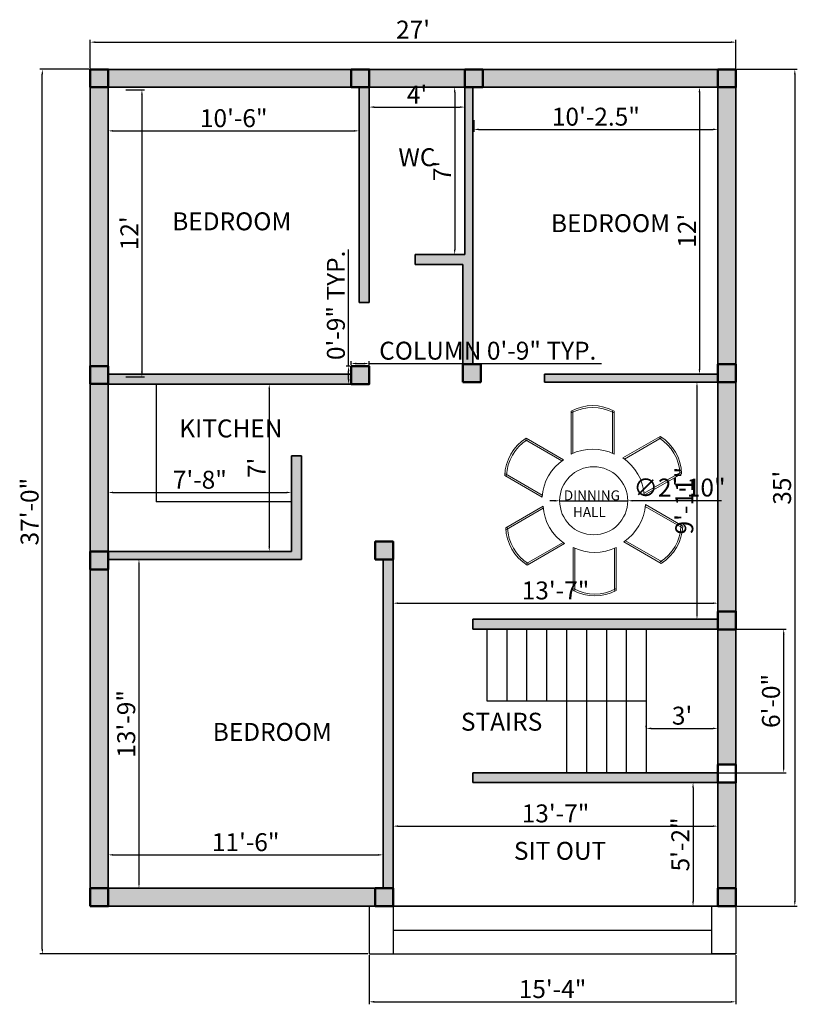
# Model space of a CAD drawing. Units: inches. Extents: x 1227 to 1617, y 420 to 915.
import ezdxf

# ---------------------------------------------------------------- set-up
doc = ezdxf.new("R2010")
doc.units = ezdxf.units.IN
for name, color, linetype, lineweight in [('A-ANNO-DIMS', 2, 'Continuous', 18), ('A-AREA-IDEN', 7, 'Continuous', 25), ('A-COLS', 7, 'Continuous', 50), ('A-FLOR-FIXT', 9, 'Continuous', 25), ('A-FLOR-STRS', 7, 'Continuous', 25), ('A-FURN', 8, 'Continuous', 18), ('A-WALL', 7, 'Continuous', 35)]:
    doc.layers.add(name, color=color, linetype=linetype, lineweight=lineweight)
doc.layers.add('A-COLS-PATT', color=18, linetype='Continuous', lineweight=13, true_color=0x000000)
doc.layers.add('A-WALL-PATT', color=114, linetype='Continuous', lineweight=13, true_color=0x139b48)
doc.styles.get("Standard").update_dxf_attribs({"font": 'arial.ttf'})
doc.dimstyles.new('ISO-25', dxfattribs={"dimtxt": 9, "dimasz": 2.5, "dimexe": 1.25, "dimexo": 0.625, "dimtad": 1, "dimlunit": 3, "dimtxsty": 'Standard', "dimcen": 2.5, "dimadec": 0, "dimazin": 0, "dimtfac": 1, "dimtmove": 0, "dimatfit": 3, "dimfxl": 1, "dimarcsym": 0})

# ---------------------------------------------------------------- blocks, each defined once
blk = doc.blocks.new('*U1')
for p, q in [((-10.82, -9.47), (-10.82, 12.17)), ((-9.92, -9.47), (-9.92, 11.75)), ((9.92, 11.75), (9.92, -9.47)), ((10.82, 12.17), (10.82, -9.47))]:
    blk.add_line(p, q)
for centre, radius, start, end in [((0, 33.94), 24.31, 243.5697, 296.4303), ((0, 10.82), 22.99, 241.9214, 298.0786), ((0, 10.82), 22.09, 241.9214, 298.0786)]:
    blk.add_arc(centre, radius, start, end)
blk = doc.blocks.new('*U2')
at = {"layer": 'A-FURN', "color": 0, "linetype": 'ByBlock', "lineweight": -2, "transparency": 16777216}
for p, rotation in [((1607.24, 674.24), 180), ((1638.29, 656.91), 120), ((1576.71, 656), 239.9999999999999), ((1577.23, 620.45), 300), ((1638.82, 621.36), 59.99999999999999)]:
    blk.add_blockref('*U1', p, dxfattribs=dict(at, rotation=rotation))
blk.add_blockref('*U1', (1608.29, 603.12), dxfattribs=at)
blk = doc.blocks.new('*D3')
at = {"layer": 'A-ANNO-DIMS', "color": 0, "lineweight": -2, "transparency": 16777216}
for p, q in [((1279.83, 879.38), (1289.21, 879.38)), ((1287.96, 876.88), (1287.96, 737.88)), ((1279.83, 735.38), (1289.21, 735.38))]:
    blk.add_line(p, q, dxfattribs=at)
at = {"layer": 'A-ANNO-DIMS', "color": 0, "transparency": 16777216}
for points in [[(1287.54, 876.88), (1288.38, 876.88), (1287.96, 879.38)], [(1287.54, 737.88), (1288.38, 737.88), (1287.96, 735.38)]]:
    blk.add_solid(points, dxfattribs=at)
at = {"layer": 'Defpoints', "color": 0, "transparency": 16777216}
for p in [(1279.2, 879.38), (1279.2, 735.38), (1287.96, 735.38)]:
    blk.add_point(p, dxfattribs=at)
at = {"layer": 'A-ANNO-DIMS', "color": 0, "transparency": 16777216, "insert": (1282.82, 807.38), "char_height": 9, "attachment_point": 5, "rotation": 90}
blk.add_mtext("12'", dxfattribs=at)
blk = doc.blocks.new('*D4')
at = {"layer": 'A-ANNO-DIMS', "color": 0, "lineweight": -2, "transparency": 16777216}
for p, q in [((1271.02, 868.89), (1271.02, 857.54)), ((1397.02, 868.89), (1397.02, 857.54)), ((1273.52, 858.79), (1394.52, 858.79))]:
    blk.add_line(p, q, dxfattribs=at)
at = {"layer": 'A-ANNO-DIMS', "color": 0, "transparency": 16777216}
for points in [[(1273.52, 859.21), (1273.52, 858.38), (1271.02, 858.79)], [(1394.52, 859.21), (1394.52, 858.38), (1397.02, 858.79)]]:
    blk.add_solid(points, dxfattribs=at)
at = {"layer": 'Defpoints', "color": 0, "transparency": 16777216}
for p in [(1271.02, 869.52), (1397.02, 869.52), (1397.02, 858.79)]:
    blk.add_point(p, dxfattribs=at)
at = {"layer": 'A-ANNO-DIMS', "color": 0, "transparency": 16777216, "insert": (1334.02, 864.01), "char_height": 9, "attachment_point": 5}
blk.add_mtext('10\'-6"', dxfattribs=at)
blk = doc.blocks.new('*D5')
at = {"layer": 'A-ANNO-DIMS', "color": 0, "lineweight": -2, "transparency": 16777216}
for p, q in [((1402.02, 880.05), (1402.02, 869.48)), ((1450.02, 880.05), (1450.02, 869.48)), ((1404.52, 870.73), (1447.52, 870.73))]:
    blk.add_line(p, q, dxfattribs=at)
at = {"layer": 'A-ANNO-DIMS', "color": 0, "transparency": 16777216}
for points in [[(1404.52, 871.15), (1404.52, 870.31), (1402.02, 870.73)], [(1447.52, 871.15), (1447.52, 870.31), (1450.02, 870.73)]]:
    blk.add_solid(points, dxfattribs=at)
at = {"layer": 'Defpoints', "color": 0, "transparency": 16777216}
for p in [(1402.02, 880.68), (1450.02, 880.68), (1450.02, 870.73)]:
    blk.add_point(p, dxfattribs=at)
at = {"layer": 'A-ANNO-DIMS', "color": 0, "transparency": 16777216, "insert": (1426.02, 875.86), "char_height": 9, "attachment_point": 5}
blk.add_mtext("4'", dxfattribs=at)
blk = doc.blocks.new('*D6')
at = {"layer": 'A-ANNO-DIMS', "color": 0, "lineweight": -2, "transparency": 16777216}
for p, q in [((1449.4, 880.68), (1443.67, 880.68)), ((1444.92, 878.18), (1444.92, 799.18)), ((1449.4, 796.68), (1443.67, 796.68))]:
    blk.add_line(p, q, dxfattribs=at)
at = {"layer": 'A-ANNO-DIMS', "color": 0, "transparency": 16777216}
for points in [[(1444.51, 878.18), (1445.34, 878.18), (1444.92, 880.68)], [(1444.51, 799.18), (1445.34, 799.18), (1444.92, 796.68)]]:
    blk.add_solid(points, dxfattribs=at)
at = {"layer": 'Defpoints', "color": 0, "transparency": 16777216}
for p in [(1450.02, 880.68), (1444.92, 796.68), (1450.02, 796.68)]:
    blk.add_point(p, dxfattribs=at)
at = {"layer": 'A-ANNO-DIMS', "color": 0, "transparency": 16777216, "insert": (1439.8, 838.68), "char_height": 9, "attachment_point": 5, "rotation": 90}
blk.add_mtext("7'", dxfattribs=at)
blk = doc.blocks.new('*D7')
at = {"layer": 'A-ANNO-DIMS', "color": 0, "lineweight": -2, "transparency": 16777216}
for p, q in [((1454.52, 864.22), (1454.52, 858.28)), ((1577.02, 864.22), (1577.02, 858.28)), ((1457.02, 859.53), (1574.52, 859.53))]:
    blk.add_line(p, q, dxfattribs=at)
at = {"layer": 'A-ANNO-DIMS', "color": 0, "transparency": 16777216}
for points in [[(1457.02, 859.95), (1457.02, 859.12), (1454.52, 859.53)], [(1574.52, 859.95), (1574.52, 859.12), (1577.02, 859.53)]]:
    blk.add_solid(points, dxfattribs=at)
at = {"layer": 'Defpoints', "color": 0, "transparency": 16777216}
for p in [(1454.52, 864.85), (1577.02, 864.85), (1577.02, 859.53)]:
    blk.add_point(p, dxfattribs=at)
at = {"layer": 'A-ANNO-DIMS', "color": 0, "transparency": 16777216, "insert": (1515.77, 864.75), "char_height": 9, "attachment_point": 5}
blk.add_mtext('10\'-2.5"', dxfattribs=at)
blk = doc.blocks.new('*D8')
at = {"layer": 'A-ANNO-DIMS', "color": 0, "lineweight": -2, "transparency": 16777216}
for p, q in [((1576.4, 880.68), (1566.51, 880.68)), ((1567.76, 878.18), (1567.76, 739.18)), ((1576.35, 736.68), (1566.51, 736.68))]:
    blk.add_line(p, q, dxfattribs=at)
at = {"layer": 'A-ANNO-DIMS', "color": 0, "transparency": 16777216}
for points in [[(1567.35, 878.18), (1568.18, 878.18), (1567.76, 880.68)], [(1567.35, 739.18), (1568.18, 739.18), (1567.76, 736.68)]]:
    blk.add_solid(points, dxfattribs=at)
at = {"layer": 'Defpoints', "color": 0, "transparency": 16777216}
for p in [(1577.02, 880.68), (1567.76, 736.68), (1576.97, 736.68)]:
    blk.add_point(p, dxfattribs=at)
at = {"layer": 'A-ANNO-DIMS', "color": 0, "transparency": 16777216, "insert": (1562.62, 808.68), "char_height": 9, "attachment_point": 5, "rotation": 90}
blk.add_mtext("12'", dxfattribs=at)
blk = doc.blocks.new('*D9')
at = {"layer": 'A-ANNO-DIMS', "color": 0, "lineweight": -2, "transparency": 16777216}
for p, q in [((1352.49, 731.68), (1353.11, 731.68)), ((1351.86, 729.18), (1351.86, 650.18)), ((1352.49, 647.68), (1353.11, 647.68))]:
    blk.add_line(p, q, dxfattribs=at)
at = {"layer": 'A-ANNO-DIMS', "color": 0, "transparency": 16777216}
for points in [[(1351.45, 729.18), (1352.28, 729.18), (1351.86, 731.68)], [(1351.45, 650.18), (1352.28, 650.18), (1351.86, 647.68)]]:
    blk.add_solid(points, dxfattribs=at)
at = {"layer": 'Defpoints', "color": 0, "transparency": 16777216}
for p in [(1351.86, 731.68), (1351.86, 647.68), (1351.86, 647.68)]:
    blk.add_point(p, dxfattribs=at)
at = {"layer": 'A-ANNO-DIMS', "color": 0, "transparency": 16777216, "insert": (1346.74, 689.68), "char_height": 9, "attachment_point": 5, "rotation": 90}
blk.add_mtext("7'", dxfattribs=at)
blk = doc.blocks.new('*D10')
at = {"layer": 'A-ANNO-DIMS', "color": 0, "lineweight": -2, "transparency": 16777216}
for p, q in [((1271.02, 674.75), (1271.02, 678.56)), ((1273.52, 677.31), (1360.52, 677.31)), ((1363.02, 674.75), (1363.02, 678.56))]:
    blk.add_line(p, q, dxfattribs=at)
at = {"layer": 'A-ANNO-DIMS', "color": 0, "transparency": 16777216}
for points in [[(1273.52, 677.73), (1273.52, 676.9), (1271.02, 677.31)], [(1360.52, 677.73), (1360.52, 676.9), (1363.02, 677.31)]]:
    blk.add_solid(points, dxfattribs=at)
at = {"layer": 'Defpoints', "color": 0, "transparency": 16777216}
for p in [(1363.02, 677.31), (1271.02, 674.12), (1363.02, 674.12)]:
    blk.add_point(p, dxfattribs=at)
at = {"layer": 'A-ANNO-DIMS', "color": 0, "transparency": 16777216, "insert": (1317.02, 682.53), "char_height": 9, "attachment_point": 5}
blk.add_mtext('7\'-8"', dxfattribs=at)
blk = doc.blocks.new('*D11')
at = {"layer": 'A-ANNO-DIMS', "color": 0, "lineweight": -2, "transparency": 16777216}
for p, q in [((1287.1, 643.68), (1287.72, 643.68)), ((1286.47, 641.18), (1286.47, 481.18)), ((1287.1, 478.68), (1287.72, 478.68))]:
    blk.add_line(p, q, dxfattribs=at)
at = {"layer": 'A-ANNO-DIMS', "color": 0, "transparency": 16777216}
for points in [[(1286.06, 641.18), (1286.89, 641.18), (1286.47, 643.68)], [(1286.06, 481.18), (1286.89, 481.18), (1286.47, 478.68)]]:
    blk.add_solid(points, dxfattribs=at)
at = {"layer": 'Defpoints', "color": 0, "transparency": 16777216}
for p in [(1286.47, 643.68), (1286.47, 478.68), (1286.47, 478.68)]:
    blk.add_point(p, dxfattribs=at)
at = {"layer": 'A-ANNO-DIMS', "color": 0, "transparency": 16777216, "insert": (1281.25, 561.18), "char_height": 9, "attachment_point": 5, "rotation": 90}
blk.add_mtext('13\'-9"', dxfattribs=at)
blk = doc.blocks.new('*D12')
at = {"layer": 'A-ANNO-DIMS', "color": 0, "lineweight": -2, "transparency": 16777216}
for p, q in [((1271.02, 491.5), (1271.02, 496.67)), ((1273.52, 495.42), (1406.52, 495.42)), ((1409.02, 491.5), (1409.02, 496.67))]:
    blk.add_line(p, q, dxfattribs=at)
at = {"layer": 'A-ANNO-DIMS', "color": 0, "transparency": 16777216}
for points in [[(1273.52, 495.84), (1273.52, 495), (1271.02, 495.42)], [(1406.52, 495.84), (1406.52, 495), (1409.02, 495.42)]]:
    blk.add_solid(points, dxfattribs=at)
at = {"layer": 'Defpoints', "color": 0, "transparency": 16777216}
for p in [(1409.02, 495.42), (1271.02, 490.87), (1409.02, 490.87)]:
    blk.add_point(p, dxfattribs=at)
at = {"layer": 'A-ANNO-DIMS', "color": 0, "transparency": 16777216, "insert": (1340.02, 500.64), "char_height": 9, "attachment_point": 5}
blk.add_mtext('11\'-6"', dxfattribs=at)
blk = doc.blocks.new('*D13')
at = {"layer": 'A-ANNO-DIMS', "color": 0, "lineweight": -2, "transparency": 16777216}
for p, q in [((1541.02, 559.52), (1541.02, 560.14)), ((1543.52, 558.89), (1574.52, 558.89)), ((1577.02, 559.52), (1577.02, 560.14))]:
    blk.add_line(p, q, dxfattribs=at)
at = {"layer": 'A-ANNO-DIMS', "color": 0, "transparency": 16777216}
for points in [[(1543.52, 559.31), (1543.52, 558.47), (1541.02, 558.89)], [(1574.52, 559.31), (1574.52, 558.47), (1577.02, 558.89)]]:
    blk.add_solid(points, dxfattribs=at)
at = {"layer": 'Defpoints', "color": 0, "transparency": 16777216}
for p in [(1541.02, 558.89), (1577.02, 558.89), (1577.02, 558.89)]:
    blk.add_point(p, dxfattribs=at)
at = {"layer": 'A-ANNO-DIMS', "color": 0, "transparency": 16777216, "insert": (1559.02, 564.11), "char_height": 9, "attachment_point": 5}
blk.add_mtext("3'", dxfattribs=at)
blk = doc.blocks.new('*D14')
at = {"layer": 'A-ANNO-DIMS', "color": 0, "lineweight": -2, "transparency": 16777216}
for p, q in [((1564.54, 529.18), (1564.54, 472.18)), ((1565.16, 531.68), (1565.79, 531.68)), ((1565.16, 469.68), (1565.79, 469.68))]:
    blk.add_line(p, q, dxfattribs=at)
at = {"layer": 'A-ANNO-DIMS', "color": 0, "transparency": 16777216}
for points in [[(1564.12, 529.18), (1564.96, 529.18), (1564.54, 531.68)], [(1564.12, 472.18), (1564.96, 472.18), (1564.54, 469.68)]]:
    blk.add_solid(points, dxfattribs=at)
at = {"layer": 'Defpoints', "color": 0, "transparency": 16777216}
for p in [(1564.54, 531.68), (1564.54, 469.68), (1564.54, 469.68)]:
    blk.add_point(p, dxfattribs=at)
at = {"layer": 'A-ANNO-DIMS', "color": 0, "transparency": 16777216, "insert": (1559.32, 500.68), "char_height": 9, "attachment_point": 5, "rotation": 90}
blk.add_mtext('5\'-2"', dxfattribs=at)
blk = doc.blocks.new('*D15')
at = {"layer": 'A-ANNO-DIMS', "color": 0, "lineweight": -2, "transparency": 16777216}
for p, q in [((1414.02, 510.47), (1414.02, 511.09)), ((1416.52, 509.84), (1574.52, 509.84)), ((1577.02, 510.47), (1577.02, 511.09))]:
    blk.add_line(p, q, dxfattribs=at)
at = {"layer": 'A-ANNO-DIMS', "color": 0, "transparency": 16777216}
for points in [[(1416.52, 510.26), (1416.52, 509.43), (1414.02, 509.84)], [(1574.52, 510.26), (1574.52, 509.43), (1577.02, 509.84)]]:
    blk.add_solid(points, dxfattribs=at)
at = {"layer": 'Defpoints', "color": 0, "transparency": 16777216}
for p in [(1414.02, 509.84), (1577.02, 509.84), (1577.02, 509.84)]:
    blk.add_point(p, dxfattribs=at)
at = {"layer": 'A-ANNO-DIMS', "color": 0, "transparency": 16777216, "insert": (1495.52, 515.07), "char_height": 9, "attachment_point": 5}
blk.add_mtext('13\'-7"', dxfattribs=at)
blk = doc.blocks.new('*D16')
at = {"layer": 'A-ANNO-DIMS', "color": 0, "lineweight": -2, "transparency": 16777216}
for p, q in [((1414.02, 633.75), (1414.02, 620.5)), ((1577.02, 633.75), (1577.02, 620.5)), ((1416.52, 621.75), (1574.52, 621.75))]:
    blk.add_line(p, q, dxfattribs=at)
at = {"layer": 'A-ANNO-DIMS', "color": 0, "transparency": 16777216}
for points in [[(1416.52, 622.16), (1416.52, 621.33), (1414.02, 621.75)], [(1574.52, 622.16), (1574.52, 621.33), (1577.02, 621.75)]]:
    blk.add_solid(points, dxfattribs=at)
at = {"layer": 'Defpoints', "color": 0, "transparency": 16777216}
for p in [(1414.02, 634.38), (1577.02, 634.38), (1577.02, 621.75)]:
    blk.add_point(p, dxfattribs=at)
at = {"layer": 'A-ANNO-DIMS', "color": 0, "transparency": 16777216, "insert": (1495.52, 626.97), "char_height": 9, "attachment_point": 5}
blk.add_mtext('13\'-7"', dxfattribs=at)
blk = doc.blocks.new('*D17')
at = {"layer": 'A-ANNO-DIMS', "color": 0, "lineweight": -2, "transparency": 16777216}
for p, q in [((1567.14, 732.68), (1567.76, 732.68)), ((1566.51, 730.18), (1566.51, 616.18)), ((1567.14, 613.68), (1567.76, 613.68))]:
    blk.add_line(p, q, dxfattribs=at)
at = {"layer": 'A-ANNO-DIMS', "color": 0, "transparency": 16777216}
for points in [[(1566.1, 730.18), (1566.93, 730.18), (1566.51, 732.68)], [(1566.1, 616.18), (1566.93, 616.18), (1566.51, 613.68)]]:
    blk.add_solid(points, dxfattribs=at)
at = {"layer": 'Defpoints', "color": 0, "transparency": 16777216}
for p in [(1566.51, 732.68), (1566.51, 613.68), (1566.51, 613.68)]:
    blk.add_point(p, dxfattribs=at)
at = {"layer": 'A-ANNO-DIMS', "color": 0, "transparency": 16777216, "insert": (1561.29, 673.18), "char_height": 9, "attachment_point": 5, "rotation": 90}
blk.add_mtext('9\'-11"', dxfattribs=at)
blk = doc.blocks.new('*D18')
at = {"layer": 'A-ANNO-DIMS', "color": 0, "lineweight": -2, "transparency": 16777216}
for p, q in [((1262.02, 890.3), (1262.02, 904.56)), ((1586.02, 890.3), (1586.02, 904.56)), ((1264.52, 903.31), (1583.52, 903.31))]:
    blk.add_line(p, q, dxfattribs=at)
at = {"layer": 'A-ANNO-DIMS', "color": 0, "transparency": 16777216}
for points in [[(1264.52, 903.73), (1264.52, 902.9), (1262.02, 903.31)], [(1583.52, 903.73), (1583.52, 902.9), (1586.02, 903.31)]]:
    blk.add_solid(points, dxfattribs=at)
at = {"layer": 'Defpoints', "color": 0, "transparency": 16777216}
for p in [(1586.02, 903.31), (1262.02, 889.68), (1586.02, 889.68)]:
    blk.add_point(p, dxfattribs=at)
at = {"layer": 'A-ANNO-DIMS', "color": 0, "transparency": 16777216, "insert": (1424.02, 908.46), "char_height": 9, "attachment_point": 5}
blk.add_mtext("27'", dxfattribs=at)
blk = doc.blocks.new('*D19')
at = {"layer": 'A-ANNO-DIMS', "color": 0, "lineweight": -2, "transparency": 16777216}
for p, q in [((1586.65, 889.68), (1616.86, 889.68)), ((1615.61, 887.18), (1615.61, 472.18)), ((1586.65, 469.68), (1616.86, 469.68))]:
    blk.add_line(p, q, dxfattribs=at)
at = {"layer": 'A-ANNO-DIMS', "color": 0, "transparency": 16777216}
for points in [[(1615.19, 887.18), (1616.02, 887.18), (1615.61, 889.68)], [(1615.19, 472.18), (1616.02, 472.18), (1615.61, 469.68)]]:
    blk.add_solid(points, dxfattribs=at)
at = {"layer": 'Defpoints', "color": 0, "transparency": 16777216}
for p in [(1586.02, 889.68), (1586.02, 469.68), (1615.61, 469.68)]:
    blk.add_point(p, dxfattribs=at)
at = {"layer": 'A-ANNO-DIMS', "color": 0, "transparency": 16777216, "insert": (1610.38, 679.68), "char_height": 9, "attachment_point": 5, "rotation": 90}
blk.add_mtext("35'", dxfattribs=at)
blk = doc.blocks.new('COLUMN-9X9-IN')
blk.add_lwpolyline([(0, 0), (9, 0), (9, 9), (0, 9)], close=True)
blk = doc.blocks.new('*D21')
at = {"layer": 'A-ANNO-DIMS', "color": 0, "lineweight": -2, "transparency": 16777216}
for p, q in [((1393.02, 741.3), (1393.02, 743.28)), ((1395.52, 742.03), (1399.52, 742.03)), ((1402.02, 741.3), (1402.02, 743.28)), ((1402.02, 742.03), (1518.51, 742.03))]:
    blk.add_line(p, q, dxfattribs=at)
at = {"layer": 'A-ANNO-DIMS', "color": 0, "transparency": 16777216}
for points in [[(1395.52, 742.44), (1395.52, 741.61), (1393.02, 742.03)], [(1399.52, 742.44), (1399.52, 741.61), (1402.02, 742.03)]]:
    blk.add_solid(points, dxfattribs=at)
at = {"layer": 'Defpoints', "color": 0, "transparency": 16777216}
for p in [(1402.02, 742.03), (1393.02, 740.68), (1402.02, 740.68)]:
    blk.add_point(p, dxfattribs=at)
at = {"layer": 'A-ANNO-DIMS', "color": 0, "transparency": 16777216, "insert": (1461.51, 747.31), "char_height": 9, "attachment_point": 5}
blk.add_mtext('COLUMN 0\'-9" TYP.', dxfattribs=at)
blk = doc.blocks.new('*D22')
at = {"layer": 'A-ANNO-DIMS', "color": 0, "lineweight": -2, "transparency": 16777216}
for p, q in [((1391.67, 740.68), (1391.67, 799.29)), ((1392.4, 740.68), (1390.42, 740.68)), ((1391.67, 734.18), (1391.67, 738.18)), ((1392.4, 731.68), (1390.42, 731.68))]:
    blk.add_line(p, q, dxfattribs=at)
at = {"layer": 'A-ANNO-DIMS', "color": 0, "transparency": 16777216}
for points in [[(1391.26, 738.18), (1392.09, 738.18), (1391.67, 740.68)], [(1391.26, 734.18), (1392.09, 734.18), (1391.67, 731.68)]]:
    blk.add_solid(points, dxfattribs=at)
at = {"layer": 'Defpoints', "color": 0, "transparency": 16777216}
for p in [(1391.67, 740.68), (1393.02, 740.68), (1393.02, 731.68)]:
    blk.add_point(p, dxfattribs=at)
at = {"layer": 'A-ANNO-DIMS', "color": 0, "transparency": 16777216, "insert": (1386.45, 771.23), "char_height": 9, "attachment_point": 5, "rotation": 90}
blk.add_mtext('0\'-9" TYP.', dxfattribs=at)
blk = doc.blocks.new('*D23')
at = {"layer": 'A-ANNO-DIMS', "color": 0, "lineweight": -2, "transparency": 16777216}
for p, q in [((1402.02, 445.05), (1402.02, 420.43)), ((1586.02, 445.05), (1586.02, 420.43)), ((1404.52, 421.68), (1583.52, 421.68))]:
    blk.add_line(p, q, dxfattribs=at)
at = {"layer": 'A-ANNO-DIMS', "color": 0, "transparency": 16777216}
for points in [[(1404.52, 422.09), (1404.52, 421.26), (1402.02, 421.68)], [(1583.52, 422.09), (1583.52, 421.26), (1586.02, 421.68)]]:
    blk.add_solid(points, dxfattribs=at)
at = {"layer": 'Defpoints', "color": 0, "transparency": 16777216}
for p in [(1402.02, 445.68), (1586.02, 445.68), (1586.02, 421.68)]:
    blk.add_point(p, dxfattribs=at)
at = {"layer": 'A-ANNO-DIMS', "color": 0, "transparency": 16777216, "insert": (1494.02, 426.9), "char_height": 9, "attachment_point": 5}
blk.add_mtext('15\'-4"', dxfattribs=at)
blk = doc.blocks.new('*D24')
at = {"layer": 'A-ANNO-DIMS', "color": 0, "lineweight": -2, "transparency": 16777216}
for p, q in [((1577.65, 608.68), (1611.27, 608.68)), ((1610.02, 539.18), (1610.02, 606.18)), ((1577.65, 536.68), (1611.27, 536.68))]:
    blk.add_line(p, q, dxfattribs=at)
at = {"layer": 'A-ANNO-DIMS', "color": 0, "transparency": 16777216}
for points in [[(1609.61, 606.18), (1610.44, 606.18), (1610.02, 608.68)], [(1609.61, 539.18), (1610.44, 539.18), (1610.02, 536.68)]]:
    blk.add_solid(points, dxfattribs=at)
at = {"layer": 'Defpoints', "color": 0, "transparency": 16777216}
for p in [(1577.02, 608.68), (1610.02, 608.68), (1577.02, 536.68)]:
    blk.add_point(p, dxfattribs=at)
at = {"layer": 'A-ANNO-DIMS', "color": 0, "transparency": 16777216, "insert": (1604.8, 572.68), "char_height": 9, "attachment_point": 5, "rotation": 90}
blk.add_mtext('6\'-0"', dxfattribs=at)
blk = doc.blocks.new('*D25')
at = {"layer": 'A-ANNO-DIMS', "color": 0, "lineweight": -2, "transparency": 16777216}
for p, q in [((1261.4, 889.68), (1236.72, 889.68)), ((1237.97, 448.18), (1237.97, 887.18)), ((1401.4, 445.68), (1236.72, 445.68))]:
    blk.add_line(p, q, dxfattribs=at)
at = {"layer": 'A-ANNO-DIMS', "color": 0, "transparency": 16777216}
for points in [[(1237.56, 887.18), (1238.39, 887.18), (1237.97, 889.68)], [(1237.56, 448.18), (1238.39, 448.18), (1237.97, 445.68)]]:
    blk.add_solid(points, dxfattribs=at)
at = {"layer": 'Defpoints', "color": 0, "transparency": 16777216}
for p in [(1237.97, 889.68), (1262.02, 889.68), (1402.02, 445.68)]:
    blk.add_point(p, dxfattribs=at)
at = {"layer": 'A-ANNO-DIMS', "color": 0, "transparency": 16777216, "insert": (1232.75, 667.68), "char_height": 9, "attachment_point": 5, "rotation": 90}
blk.add_mtext('37\'-0"', dxfattribs=at)
blk = doc.blocks.new('*D26')
at = {"layer": 'A-ANNO-DIMS', "color": 0, "lineweight": -2, "transparency": 16777216}
for p, q in [((1495.09, 673.15), (1492.59, 673.15)), ((1497.59, 673.15), (1531.78, 673.15)), ((1578.74, 673.15), (1534.28, 673.15))]:
    blk.add_line(p, q, dxfattribs=at)
at = {"layer": 'A-ANNO-DIMS', "color": 0, "transparency": 16777216}
for points in [[(1495.09, 673.57), (1495.09, 672.73), (1497.59, 673.15)], [(1534.28, 673.57), (1534.28, 672.73), (1531.78, 673.15)]]:
    blk.add_solid(points, dxfattribs=at)
at = {"layer": 'Defpoints', "color": 0, "transparency": 16777216}
for p in [(1497.59, 673.15), (1531.78, 673.15)]:
    blk.add_point(p, dxfattribs=at)
at = {"layer": 'A-ANNO-DIMS', "color": 0, "transparency": 16777216, "insert": (1557.76, 678.62), "char_height": 9, "attachment_point": 5, "rotation": 0.001}
blk.add_mtext('∅2\'-10"', dxfattribs=at)

msp = doc.modelspace()

# ---------------------------------------------------------------- hatches: boundary and pattern name
at = {"layer": 'A-COLS-PATT'}
h = msp.add_hatch(color=256, dxfattribs=at)
h.dxf.hatch_style = 1
h.paths.add_polyline_path([(1271.023, 889.677), (1262.023, 889.677), (1262.023, 880.677), (1271.023, 880.677)])
h = msp.add_hatch(color=256, dxfattribs=at)
h.dxf.hatch_style = 1
h.paths.add_polyline_path([(1271.023, 478.677), (1262.023, 478.677), (1262.023, 469.677), (1271.023, 469.677)])
h.paths.add_polyline_path([(1414.023, 478.677), (1405.023, 478.677), (1405.023, 469.677), (1414.023, 469.677)])
h.paths.add_polyline_path([(1271.023, 647.677), (1262.023, 647.677), (1262.023, 638.677), (1271.023, 638.677)])
h.paths.add_polyline_path([(1402.023, 889.677), (1393.023, 889.677), (1393.023, 880.677), (1402.023, 880.677)])
h.paths.add_polyline_path([(1459.023, 889.677), (1450.023, 889.677), (1450.023, 880.677), (1459.023, 880.677)])
h.paths.add_polyline_path([(1586.023, 889.677), (1577.023, 889.677), (1577.023, 880.677), (1586.023, 880.677)])
h.paths.add_polyline_path([(1585.974, 741.727), (1577.023, 741.727), (1577.023, 736.677), (1576.974, 732.727), (1585.974, 732.727)])
h.paths.add_polyline_path([(1586.023, 617.607), (1577.023, 617.607), (1577.023, 608.607), (1586.023, 608.607)])
h.paths.add_polyline_path([(1414.023, 652.677), (1405.023, 652.677), (1405.023, 643.677), (1414.023, 643.677)])
h.paths.add_polyline_path([(1402.023, 740.677), (1393.023, 740.677), (1393.023, 731.677), (1402.023, 731.677)])
h.paths.add_polyline_path([(1458.015, 741.677), (1449.023, 741.677), (1449.023, 732.677), (1458.015, 732.677)])
h.paths.add_polyline_path([(1586.023, 478.677), (1577.023, 478.677), (1577.023, 469.677), (1586.023, 469.677)])
h.paths.add_polyline_path([(1270.972, 740.755), (1262.023, 740.755), (1262.023, 731.755), (1270.972, 731.755)])
at = {"layer": 'A-WALL-PATT'}
h = msp.add_hatch(color=256, dxfattribs=at)
h.dxf.hatch_style = 1
h.paths.add_polyline_path([(1262.023, 740.755), (1271.023, 740.755), (1271.023, 880.677), (1262.023, 880.677)])
h.paths.add_polyline_path([(1450.023, 880.677), (1450.023, 889.677), (1402.023, 889.677), (1402.023, 880.677)])
h.paths.add_polyline_path([(1577.023, 880.677), (1577.023, 889.677), (1459.023, 889.677), (1459.023, 880.677)])
h.paths.add_polyline_path([(1292.251, 796.549), (1292.251, 817.434), (1273.705, 817.434), (1273.705, 796.549)], flags=9)
h.paths.add_polyline_path([(1491.876, 855.398), (1538.89, 855.398), (1538.89, 873.944), (1491.876, 873.944)], flags=9)
h = msp.add_hatch(color=256, dxfattribs=at)
h.dxf.hatch_style = 1
h.paths.add_polyline_path([(1393.023, 889.677), (1271.023, 889.677), (1271.023, 880.677), (1393.023, 880.677)])
h.paths.add_polyline_path([(1393.023, 736.677), (1270.972, 736.677), (1270.972, 731.677), (1393.023, 731.677)])
h.paths.add_polyline_path([(1271.023, 731.677), (1270.972, 731.677), (1262.023, 731.754), (1262.023, 647.677), (1271.023, 647.677)])
h.paths.add_polyline_path([(1402.023, 880.677), (1397.023, 880.677), (1397.023, 772.677), (1402.023, 772.677)])
h.paths.add_polyline_path([(1454.023, 880.677), (1450.023, 880.677), (1450.023, 796.677), (1425.023, 796.677), (1425.023, 791.677), (1449.023, 791.677), (1449.023, 741.677), (1454.023, 741.677)])
h.paths.add_polyline_path([(1576.974, 736.677), (1490.023, 736.677), (1490.023, 732.677), (1576.974, 732.677)])
h.paths.add_polyline_path([(1586.023, 880.677), (1577.023, 880.677), (1577.023, 741.727), (1586.023, 741.727)])
h.paths.add_polyline_path([(1586.023, 608.607), (1577.023, 608.607), (1577.023, 540.743), (1586.023, 540.743)])
h.paths.add_polyline_path([(1586.023, 732.727), (1577.023, 732.727), (1577.023, 617.607), (1586.023, 617.607)])
h.paths.add_polyline_path([(1577.023, 613.677), (1454.023, 613.677), (1454.023, 608.677), (1577.023, 608.677)])
h.paths.add_polyline_path([(1577.023, 536.677), (1454.023, 536.677), (1454.023, 531.677), (1577.023, 531.677), (1577.023, 531.743)])
h.paths.add_polyline_path([(1586.023, 531.743), (1577.023, 531.743), (1577.023, 531.677), (1577.023, 478.677), (1586.023, 478.677)])
h.paths.add_polyline_path([(1405.023, 478.677), (1271.023, 478.677), (1271.023, 469.677), (1405.023, 469.677)])
h.paths.add_polyline_path([(1414.023, 643.677), (1409.023, 643.677), (1409.023, 478.677), (1414.023, 478.677)])
h.paths.add_polyline_path([(1271.023, 638.677), (1262.023, 638.677), (1262.023, 478.677), (1271.023, 478.677)])
h.paths.add_polyline_path([(1368.023, 695.677), (1363.023, 695.677), (1363.023, 647.677), (1271.023, 647.677), (1271.023, 643.677), (1367.023, 643.677), (1368.023, 643.677), (1368.023, 644.677)])

# ---------------------------------------------------------------- linework, layer by layer
at = {"layer": 'A-FLOR-FIXT'}
for p in [(1295.023, 731.677), (1363.023, 672.677)]:
    msp.add_line(p, (1295.023, 672.677), dxfattribs=at)
at = {"layer": 'A-FLOR-STRS'}
for p, q in [((1461.023, 608.677), (1461.023, 572.677)), ((1471.023, 608.677), (1471.023, 572.677)), ((1481.023, 608.677), (1481.023, 572.677)), ((1491.023, 608.677), (1491.023, 572.677)), ((1501.023, 608.677), (1501.023, 536.677)), ((1511.023, 608.677), (1511.023, 536.677)), ((1521.023, 608.677), (1521.023, 536.677)), ((1531.023, 608.677), (1531.023, 536.677)), ((1541.023, 608.677), (1541.023, 536.677)), ((1461.023, 572.677), (1541.023, 572.677)), ((1402.023, 469.677), (1402.023, 445.677)), ((1414.023, 469.677), (1414.023, 445.677)), ((1574.023, 445.677), (1574.023, 469.677)), ((1586.023, 469.677), (1586.023, 445.677)), ((1414.023, 457.677), (1574.023, 457.677)), ((1402.023, 445.677), (1426.023, 445.677)), ((1414.023, 445.677), (1586.023, 445.677)), ((1586.023, 445.677), (1574.023, 445.677))]:
    msp.add_line(p, q, dxfattribs=at)
at = {"layer": 'A-FURN'}
msp.add_circle((1514.683, 673.15), 17.097, dxfattribs=at)
at = {"layer": 'A-WALL'}
for p, q in [((1586.023, 889.677), (1262.023, 889.677)), ((1262.023, 889.677), (1262.023, 469.677)), ((1586.023, 469.677), (1586.023, 889.677)), ((1271.023, 880.677), (1271.023, 736.677)), ((1397.023, 880.677), (1271.023, 880.677)), ((1397.023, 880.677), (1397.023, 772.677)), ((1402.023, 880.677), (1402.023, 772.677)), ((1450.023, 880.677), (1402.023, 880.677)), ((1450.023, 880.677), (1450.023, 796.677)), ((1577.023, 880.677), (1454.023, 880.677)), ((1454.023, 880.677), (1454.023, 741.677)), ((1577.023, 736.677), (1577.023, 880.677)), ((1425.023, 796.677), (1449.023, 796.677)), ((1450.023, 796.677), (1425.023, 796.677)), ((1425.023, 796.677), (1425.023, 791.677)), ((1425.023, 791.677), (1449.023, 791.677)), ((1449.023, 791.677), (1449.023, 732.677)), ((1397.023, 772.677), (1402.023, 772.677)), ((1393.023, 736.677), (1271.023, 736.677)), ((1402.023, 731.677), (1402.023, 736.677)), ((1402.023, 736.677), (1402.023, 736.677)), ((1577.023, 736.677), (1490.023, 736.677)), ((1490.023, 736.677), (1490.023, 732.677)), ((1401.023, 731.677), (1271.023, 731.677)), ((1271.023, 731.677), (1271.023, 647.677)), ((1401.023, 731.677), (1402.023, 731.677)), ((1449.023, 732.677), (1454.023, 732.677)), ((1577.023, 732.677), (1490.023, 732.677)), ((1577.023, 613.677), (1577.023, 732.677)), ((1363.023, 695.677), (1363.023, 647.677)), ((1368.023, 695.677), (1363.023, 695.677)), ((1368.023, 695.677), (1368.023, 644.677)), ((1363.023, 647.677), (1271.023, 647.677)), ((1367.023, 643.677), (1271.023, 643.677)), ((1271.023, 643.677), (1271.023, 478.677)), ((1367.023, 643.677), (1368.023, 643.677)), ((1368.023, 643.677), (1368.023, 644.677)), ((1409.023, 643.677), (1409.023, 478.677)), ((1414.023, 643.677), (1409.023, 643.677)), ((1414.023, 643.677), (1414.023, 469.677)), ((1577.023, 613.677), (1454.023, 613.677)), ((1454.023, 613.677), (1454.023, 608.677)), ((1577.023, 608.677), (1454.023, 608.677)), ((1577.023, 536.677), (1577.023, 608.677)), ((1577.023, 536.677), (1454.023, 536.677)), ((1454.023, 536.677), (1454.023, 531.677)), ((1577.023, 531.677), (1454.023, 531.677)), ((1577.023, 469.677), (1577.023, 531.677)), ((1271.023, 478.677), (1409.023, 478.677)), ((1262.023, 469.677), (1586.023, 469.677))]:
    msp.add_line(p, q, dxfattribs=at)

# ---------------------------------------------------------------- block references
at = {"layer": 'A-COLS'}
for p in [(1262.023, 880.677), (1393.023, 880.677), (1450.023, 880.677), (1577.023, 880.677), (1449.015, 732.677), (1576.974, 732.728), (1261.972, 731.755), (1393.022, 731.677), (1405.023, 643.677), (1262.023, 638.677), (1577.023, 608.607), (1577.023, 531.743), (1262.023, 469.677), (1405.023, 469.677), (1577.023, 469.677)]:
    msp.add_blockref('COLUMN-9X9-IN', p, dxfattribs=at)
at = {"layer": 'A-FURN'}
msp.add_blockref('*U2', (-93.078, 34.469), dxfattribs=at)

# ---------------------------------------------------------------- texts
at = {"layer": 'A-AREA-IDEN', "attachment_point": 1}
for s, width, insert, char_height in [('WC', 32.3639, (1416.659, 850.062), 9), ('BEDROOM', 69.18881, (1303.19, 817.895), 9), ('BEDROOM', 69.18881, (1493.228, 816.973), 9), ('KITCHEN', 20.10174, (1306.713, 713.952), 9), ('DINNING \\P   HALL', 36.51835, (1499.688, 678.355), 5), ('STAIRS', 28.3595, (1448.036, 566.757), 9), ('BEDROOM', 69.18881, (1323.485, 561.638), 9), ('SIT OUT', 79.99258, (1474.636, 501.953), 9)]:
    msp.add_mtext_dynamic_manual_height_columns(s, width=width, gutter_width=12.5, heights=[0], dxfattribs=dict(at, insert=insert, char_height=char_height))

# ---------------------------------------------------------------- dimensions: what is measured, and where the dimension line sits
at = {"layer": 'A-ANNO-DIMS'}
for base, p1, p2, override, picture, middle in [((1586.023, 903.315), (1262.023, 889.677), (1586.023, 889.677), {"dimclrd": 0, "dimclre": 0, "dimclrt": 0}, '*D18', (1424.023, 908.458)), ((1450.023, 870.731), (1402.023, 880.677), (1450.023, 880.677), {"dimclrd": 0, "dimclre": 0, "dimclrt": 0}, '*D5', (1426.023, 875.856)), ((1397.023, 858.793), (1271.023, 869.517), (1397.023, 869.517), {"dimclrd": 0, "dimclre": 0, "dimclrt": 0}, '*D4', (1334.023, 864.014)), ((1577.023, 859.534), (1454.523, 864.85), (1577.023, 864.85), {"dimclrd": 0, "dimclre": 0, "dimclrt": 0}, '*D7', (1515.773, 864.754)), ((1363.023, 677.312), (1271.023, 674.122), (1363.023, 674.122), {"dimclrd": 0, "dimclre": 0, "dimclrt": 0}, '*D10', (1317.023, 682.532)), ((1577.023, 621.747), (1414.023, 634.377), (1577.023, 634.377), {"dimclrd": 0, "dimclre": 0, "dimclrt": 0}, '*D16', (1495.523, 626.97)), ((1577.023, 558.891), (1541.023, 558.891), (1577.023, 558.891), {"dimclrd": 0, "dimclre": 0, "dimclrt": 0}, '*D13', (1559.023, 564.114)), ((1577.023, 509.843), (1414.023, 509.843), (1577.023, 509.843), {"dimclrd": 0, "dimclre": 0, "dimclrt": 0}, '*D15', (1495.523, 515.066)), ((1409.023, 495.42), (1271.023, 490.872), (1409.023, 490.872), {"dimclrd": 0, "dimclre": 0, "dimclrt": 0}, '*D12', (1340.023, 500.641)), ((1586.023, 421.677), (1402.023, 445.677), (1586.023, 445.677), {"dimdec": 1, "dimlfac": 1, "dimrnd": 0, "dimzin": 1, "dimdsep": 46, "dimlunit": 4, "dimfrac": 2}, '*D23', (1494.023, 426.897))]:
    dim = msp.add_linear_dim(base=base, p1=p1, p2=p2, dimstyle='ISO-25', override=override, dxfattribs=at)
    dim.commit()
    dim.dimension.update_dxf_attribs({"geometry": picture, "text_midpoint": middle})
for base, p1, p2, override, picture, middle in [((1237.972, 889.677), (1402.023, 445.677), (1262.023, 889.677), {"dimdec": 1, "dimlfac": 1, "dimrnd": 0, "dimzin": 1, "dimdsep": 46, "dimlunit": 4, "dimfrac": 2}, '*D25', (1232.749, 667.677)), ((1615.607, 469.677), (1586.023, 889.677), (1586.023, 469.677), {"dimclrd": 0, "dimclre": 0, "dimclrt": 0}, '*D19', (1610.384, 679.677)), ((1444.924, 796.677), (1450.023, 880.677), (1450.023, 796.677), {"dimclrd": 0, "dimclre": 0, "dimclrt": 0}, '*D6', (1439.799, 838.677)), ((1567.764, 736.677), (1577.023, 880.677), (1576.974, 736.677), {"dimclrd": 0, "dimclre": 0, "dimclrt": 0}, '*D8', (1562.621, 808.677)), ((1287.962, 735.382), (1279.204, 879.382), (1279.204, 735.382), {"dimclrd": 0, "dimclre": 0, "dimclrt": 0}, '*D3', (1282.818, 807.382)), ((1351.863, 647.677), (1351.863, 731.677), (1351.863, 647.677), {"dimclrd": 0, "dimclre": 0, "dimclrt": 0}, '*D9', (1346.738, 689.677)), ((1566.514, 613.677), (1566.514, 732.677), (1566.514, 613.677), {"dimclrd": 0, "dimclre": 0, "dimclrt": 0}, '*D17', (1561.294, 673.177)), ((1286.473, 478.677), (1286.473, 643.677), (1286.473, 478.677), {"dimclrd": 0, "dimclre": 0, "dimclrt": 0}, '*D11', (1281.25, 561.177)), ((1610.023, 608.677), (1577.023, 536.677), (1577.023, 608.677), {"dimdec": 1, "dimlfac": 1, "dimrnd": 0, "dimzin": 1, "dimdsep": 46, "dimlunit": 4, "dimfrac": 2}, '*D24', (1604.803, 572.677)), ((1564.54, 469.677), (1564.54, 531.677), (1564.54, 469.677), {"dimclrd": 0, "dimclre": 0, "dimclrt": 0}, '*D14', (1559.319, 500.677))]:
    dim = msp.add_linear_dim(base=base, p1=p1, p2=p2, angle=90, dimstyle='ISO-25', override=override, dxfattribs=at)
    dim.commit()
    dim.dimension.update_dxf_attribs({"geometry": picture, "text_midpoint": middle})
dim = msp.add_linear_dim(base=(1391.673, 740.677), p1=(1393.023, 731.677), p2=(1393.023, 740.677), angle=90, text='<> TYP.', dimstyle='ISO-25', override={"dimdec": 1, "dimlfac": 1, "dimrnd": 0, "dimzin": 1, "dimdsep": 46, "dimlunit": 4, "dimfrac": 2}, dxfattribs=at)
dim.commit()
dim.dimension.update_dxf_attribs({"geometry": '*D22', "text_midpoint": (1386.452, 771.231)})
dim = msp.add_linear_dim(base=(1402.023, 742.027), p1=(1393.023, 740.677), p2=(1402.023, 740.677), text='COLUMN <> TYP.', dimstyle='ISO-25', override={"dimdec": 1, "dimlfac": 1, "dimrnd": 0, "dimzin": 1, "dimdsep": 46, "dimlunit": 4, "dimfrac": 2}, dxfattribs=at)
dim.commit()
dim.dimension.update_dxf_attribs({"geometry": '*D21', "text_midpoint": (1461.514, 747.308)})
dim = msp.add_diameter_dim_2p(p1=(1497.586, 673.149), p2=(1531.78, 673.15), dimstyle='ISO-25', override={"dimdec": 1, "dimlfac": 1, "dimrnd": 0, "dimzin": 1, "dimdsep": 46, "dimlunit": 4, "dimfrac": 2}, dxfattribs=at)
dim.commit()
dim.dimension.update_dxf_attribs({"geometry": '*D26', "text_midpoint": (1557.76, 673.15)})

doc.saveas('drawing.dxf')
